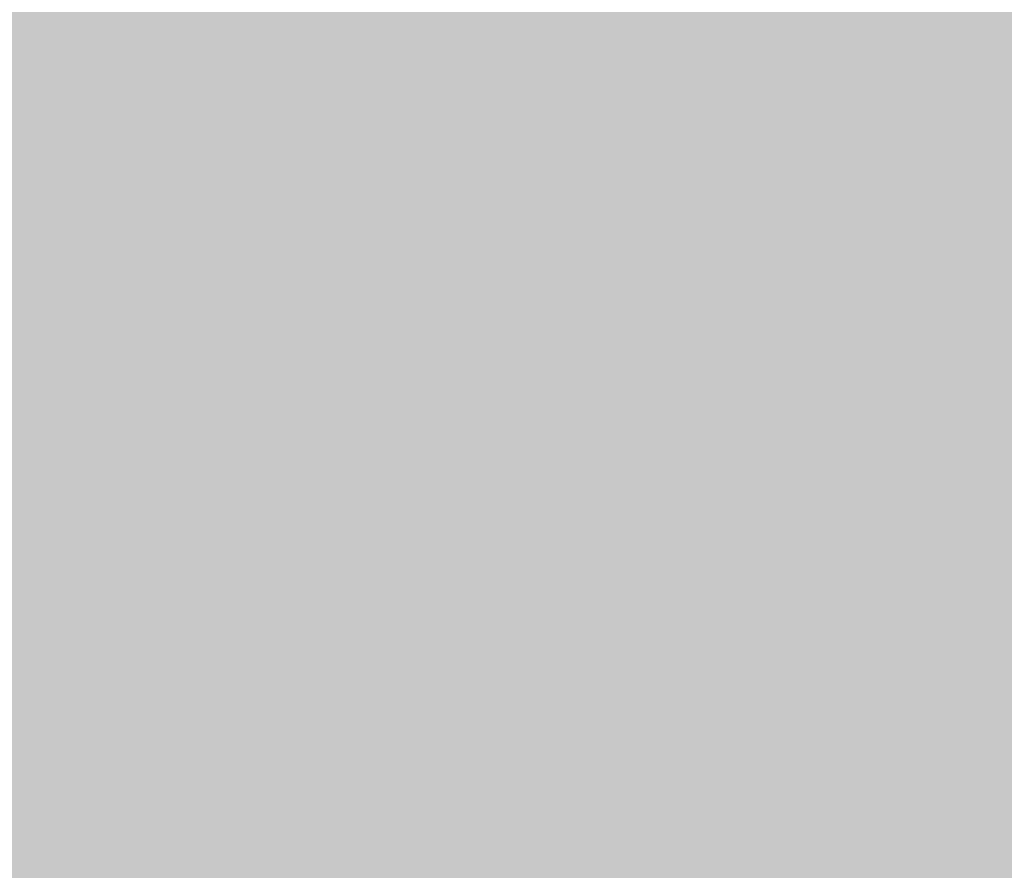
# Model space of a CAD drawing. Units: millimetres. Extents: x -22994 to 29398, y -19990 to 20176.
# Tile 66 of 135: x 225.8137 to 226.3549, y 83.796 to 84.2638. Entities that reach past the tile are written whole.
import ezdxf
from ezdxf import colors
from ezdxf.entities.mleader import LeaderData, LeaderLine
from ezdxf.math import Vec2, Vec3

# ---------------------------------------------------------------- set-up
doc = ezdxf.new("R2010")
doc.units = ezdxf.units.MM
doc.header["$MEASUREMENT"] = 0
for name, color, linetype, lineweight in [('M-ANNO-TEXT', 7, 'Continuous', 25), ('M-DIMS', 2, 'Continuous', 18), ('M-EQPM-PATT', 7, 'Continuous', 18)]:
    doc.layers.add(name, color=color, linetype=linetype, lineweight=lineweight)
doc.styles.get("Standard").update_dxf_attribs({"font": 'arial.ttf'})
doc.dimstyles.get("Standard").update_dxf_attribs({"dimtxt": 0.18, "dimasz": 10000, "dimexe": 0.18, "dimexo": 0.0625, "dimgap": 0.09, "dimtad": 0, "dimtih": 1, "dimtoh": 1, "dimdec": 0, "dimzin": 0, "dimdsep": 46, "dimtxsty": 'Standard', "dimcen": 0.09, "dimadec": 0, "dimazin": 0, "dimtfac": 1, "dimtdec": 0, "dimtofl": 0, "dimtmove": 0, "dimatfit": 3, "dimfxl": 1, "dimtolj": 1, "dimtzin": 0, "dimlwd": 30, "dimarcsym": 0})

# ---------------------------------------------------------------- blocks, each defined once
blk = doc.blocks.new('*D2')
at = {"layer": 'Defpoints', "color": 0, "transparency": 16777216}
for p in [(6.67733, 10.27127), (290.85202, 10.27127), (290.85202, -5.07873)]:
    blk.add_point(p, dxfattribs=at)
at = {"layer": 'M-DIMS', "color": 0, "lineweight": -2, "transparency": 16777216}
for p, q in [((6.67733, 10.20877), (6.67733, -5.25873)), ((290.85202, 10.20877), (290.85202, -5.25873))]:
    blk.add_line(p, q, dxfattribs=at)
at = {"layer": 'M-DIMS', "color": 0, "lineweight": 30, "transparency": 16777216}
for p, q in [((-9993.32267, -5.07873), (-19993.32267, -5.07873)), ((10290.85202, -5.07873), (20290.85202, -5.07873))]:
    blk.add_line(p, q, dxfattribs=at)
at = {"layer": 'M-DIMS', "color": 0, "transparency": 16777216}
for points in [[(-9993.32267, 1661.58794), (-9993.32267, -1671.74539), (6.67733, -5.07873)], [(10290.85202, 1661.58794), (10290.85202, -1671.74539), (290.85202, -5.07873)]]:
    blk.add_solid(points, dxfattribs=at)
at = {"layer": 'M-DIMS', "color": 0, "transparency": 16777216, "insert": (148.76467, -5.07873), "char_height": 0.18, "attachment_point": 5}
blk.add_mtext('\\A1;284.2', dxfattribs=at)
blk = doc.blocks.new('*D3')
at = {"layer": 'Defpoints', "color": 0, "transparency": 16777216}
for p in [(110.26467, 204.16539), (110.26467, 176.36616), (95.83267, 127.96702)]:
    blk.add_point(p, dxfattribs=at)
at = {"layer": 'M-DIMS', "color": 0, "lineweight": -2, "transparency": 16777216}
for p, q in [((95.83267, 128.02952), (95.83267, 204.34539)), ((110.26467, 176.42866), (110.26467, 204.34539))]:
    blk.add_line(p, q, dxfattribs=at)
at = {"layer": 'M-DIMS', "color": 0, "lineweight": 30, "transparency": 16777216}
for p, q in [((-9904.16734, 204.16539), (-19904.16733, 204.16539)), ((10110.26467, 204.16539), (20110.26467, 204.16539))]:
    blk.add_line(p, q, dxfattribs=at)
at = {"layer": 'M-DIMS', "color": 0, "transparency": 16777216}
for points in [[(-9904.16734, 1870.83206), (-9904.16734, -1462.50127), (95.83267, 204.16539)], [(10110.26467, 1870.83206), (10110.26467, -1462.50127), (110.26467, 204.16539)]]:
    blk.add_solid(points, dxfattribs=at)
at = {"layer": 'M-DIMS', "color": 0, "transparency": 16777216, "insert": (103.04867, 204.16539), "char_height": 0.18, "attachment_point": 5}
blk.add_mtext('\\A1;14.432', dxfattribs=at)
blk = doc.blocks.new('*D4')
at = {"layer": 'Defpoints', "color": 0, "transparency": 16777216}
for p in [(116.26467, 204.16539), (110.26467, 176.36616), (116.26467, 176.36616)]:
    blk.add_point(p, dxfattribs=at)
at = {"layer": 'M-DIMS', "color": 0, "lineweight": -2, "transparency": 16777216}
for p, q in [((110.26467, 176.42866), (110.26467, 204.34539)), ((116.26467, 176.42866), (116.26467, 204.34539))]:
    blk.add_line(p, q, dxfattribs=at)
at = {"layer": 'M-DIMS', "color": 0, "lineweight": 30, "transparency": 16777216}
for p, q in [((-9889.73533, 204.16539), (-19889.73533, 204.16539)), ((10116.26467, 204.16539), (20116.26467, 204.16539))]:
    blk.add_line(p, q, dxfattribs=at)
at = {"layer": 'M-DIMS', "color": 0, "transparency": 16777216}
for points in [[(-9889.73533, 1870.83206), (-9889.73533, -1462.50127), (110.26467, 204.16539)], [(10116.26467, 1870.83206), (10116.26467, -1462.50127), (116.26467, 204.16539)]]:
    blk.add_solid(points, dxfattribs=at)
at = {"layer": 'M-DIMS', "color": 0, "transparency": 16777216, "insert": (113.26467, 204.16539), "char_height": 0.18, "attachment_point": 5}
blk.add_mtext('\\A1;6', dxfattribs=at)
blk = doc.blocks.new('*D5')
at = {"layer": 'Defpoints', "color": 0, "transparency": 16777216}
for p in [(181.26467, 204.16539), (116.26467, 176.36616), (181.26467, 176.36616)]:
    blk.add_point(p, dxfattribs=at)
at = {"layer": 'M-DIMS', "color": 0, "lineweight": -2, "transparency": 16777216}
for p, q in [((116.26467, 176.42866), (116.26467, 204.34539)), ((181.26467, 176.42866), (181.26467, 204.34539))]:
    blk.add_line(p, q, dxfattribs=at)
at = {"layer": 'M-DIMS', "color": 0, "lineweight": 30, "transparency": 16777216}
for p, q in [((-9883.73533, 204.16539), (-19883.73533, 204.16539)), ((10181.26467, 204.16539), (20181.26467, 204.16539))]:
    blk.add_line(p, q, dxfattribs=at)
at = {"layer": 'M-DIMS', "color": 0, "transparency": 16777216}
for points in [[(-9883.73533, 1870.83206), (-9883.73533, -1462.50127), (116.26467, 204.16539)], [(10181.26467, 1870.83206), (10181.26467, -1462.50127), (181.26467, 204.16539)]]:
    blk.add_solid(points, dxfattribs=at)
at = {"layer": 'M-DIMS', "color": 0, "transparency": 16777216, "insert": (148.76467, 204.16539), "char_height": 0.18, "attachment_point": 5}
blk.add_mtext('\\A1;65', dxfattribs=at)
blk = doc.blocks.new('*D6')
at = {"layer": 'Defpoints', "color": 0, "transparency": 16777216}
for p in [(187.26467, 204.16539), (181.26467, 176.36616), (187.26467, 176.36616)]:
    blk.add_point(p, dxfattribs=at)
at = {"layer": 'M-DIMS', "color": 0, "lineweight": -2, "transparency": 16777216}
for p, q in [((181.26467, 176.42866), (181.26467, 204.34539)), ((187.26467, 176.42866), (187.26467, 204.34539))]:
    blk.add_line(p, q, dxfattribs=at)
at = {"layer": 'M-DIMS', "color": 0, "lineweight": 30, "transparency": 16777216}
for p, q in [((-9818.73533, 204.16539), (-19818.73533, 204.16539)), ((10187.26467, 204.16539), (20187.26467, 204.16539))]:
    blk.add_line(p, q, dxfattribs=at)
at = {"layer": 'M-DIMS', "color": 0, "transparency": 16777216}
for points in [[(-9818.73533, 1870.83206), (-9818.73533, -1462.50127), (181.26467, 204.16539)], [(10187.26467, 1870.83206), (10187.26467, -1462.50127), (187.26467, 204.16539)]]:
    blk.add_solid(points, dxfattribs=at)
at = {"layer": 'M-DIMS', "color": 0, "transparency": 16777216, "insert": (184.26467, 204.16539), "char_height": 0.18, "attachment_point": 5}
blk.add_mtext('\\A1;6', dxfattribs=at)
blk = doc.blocks.new('*D7')
at = {"layer": 'Defpoints', "color": 0, "transparency": 16777216}
for p in [(201.69668, 204.16539), (187.26467, 176.36616), (201.69668, 127.96702)]:
    blk.add_point(p, dxfattribs=at)
at = {"layer": 'M-DIMS', "color": 0, "lineweight": -2, "transparency": 16777216}
for p, q in [((187.26467, 176.42866), (187.26467, 204.34539)), ((201.69668, 128.02952), (201.69668, 204.34539))]:
    blk.add_line(p, q, dxfattribs=at)
at = {"layer": 'M-DIMS', "color": 0, "lineweight": 30, "transparency": 16777216}
for p, q in [((-9812.73533, 204.16539), (-19812.73533, 204.16539)), ((10201.69668, 204.16539), (20201.69668, 204.16539))]:
    blk.add_line(p, q, dxfattribs=at)
at = {"layer": 'M-DIMS', "color": 0, "transparency": 16777216}
for points in [[(-9812.73533, 1870.83206), (-9812.73533, -1462.50127), (187.26467, 204.16539)], [(10201.69668, 1870.83206), (10201.69668, -1462.50127), (201.69668, 204.16539)]]:
    blk.add_solid(points, dxfattribs=at)
at = {"layer": 'M-DIMS', "color": 0, "transparency": 16777216, "insert": (194.48068, 204.16539), "char_height": 0.18, "attachment_point": 5}
blk.add_mtext('\\A1;14.432', dxfattribs=at)
blk = doc.blocks.new('*D8')
at = {"layer": 'Defpoints', "color": 0, "transparency": 16777216}
for p in [(227.64848, 204.16539), (227.64848, 146.72957), (201.69668, 127.96702)]:
    blk.add_point(p, dxfattribs=at)
at = {"layer": 'M-DIMS', "color": 0, "lineweight": -2, "transparency": 16777216}
for p, q in [((201.69668, 128.02952), (201.69668, 204.34539)), ((227.64848, 146.79207), (227.64848, 204.34539))]:
    blk.add_line(p, q, dxfattribs=at)
at = {"layer": 'M-DIMS', "color": 0, "lineweight": 30, "transparency": 16777216}
for p, q in [((-9798.30332, 204.16539), (-19798.30332, 204.16539)), ((10227.64848, 204.16539), (20227.64848, 204.16539))]:
    blk.add_line(p, q, dxfattribs=at)
at = {"layer": 'M-DIMS', "color": 0, "transparency": 16777216}
for points in [[(-9798.30332, 1870.83206), (-9798.30332, -1462.50127), (201.69668, 204.16539)], [(10227.64848, 1870.83206), (10227.64848, -1462.50127), (227.64848, 204.16539)]]:
    blk.add_solid(points, dxfattribs=at)
at = {"layer": 'M-DIMS', "color": 0, "transparency": 16777216, "insert": (214.67258, 204.16539), "char_height": 0.18, "attachment_point": 5}
blk.add_mtext('\\A1;25.95', dxfattribs=at)
blk = doc.blocks.new('*D9')
at = {"layer": 'Defpoints', "color": 0, "transparency": 16777216}
for p in [(187.26467, 176.36616), (306.20202, 176.36616), (290.85202, 10.27127)]:
    blk.add_point(p, dxfattribs=at)
at = {"layer": 'M-DIMS', "color": 0, "lineweight": 30, "transparency": 16777216}
for p, q in [((306.20202, 10176.36616), (306.20202, 20176.36616)), ((306.20202, -9989.72873), (306.20202, -19989.72873))]:
    blk.add_line(p, q, dxfattribs=at)
at = {"layer": 'M-DIMS', "color": 0, "lineweight": -2, "transparency": 16777216}
for p, q in [((187.32717, 176.36616), (306.38202, 176.36616)), ((290.91452, 10.27127), (306.38202, 10.27127))]:
    blk.add_line(p, q, dxfattribs=at)
at = {"layer": 'M-DIMS', "color": 0, "transparency": 16777216}
for points in [[(-1360.46465, 10176.36616), (1972.86869, 10176.36616), (306.20202, 176.36616)], [(-1360.46465, -9989.72873), (1972.86869, -9989.72873), (306.20202, 10.27127)]]:
    blk.add_solid(points, dxfattribs=at)
at = {"layer": 'M-DIMS', "color": 0, "transparency": 16777216, "insert": (306.20202, 93.31872), "char_height": 0.18, "attachment_point": 5}
blk.add_mtext('\\A1;166.1', dxfattribs=at)
blk = doc.blocks.new('*D10')
at = {"layer": 'Defpoints', "color": 0, "transparency": 16777216}
for p in [(125.64978, 136.0713), (133.34587, 136.0713), (133.34587, -5.07873)]:
    blk.add_point(p, dxfattribs=at)
at = {"layer": 'M-DIMS', "color": 0, "lineweight": -2, "transparency": 16777216}
for p, q in [((125.64978, 136.0088), (125.64978, -5.25872)), ((133.34587, 136.0088), (133.34587, -5.25872))]:
    blk.add_line(p, q, dxfattribs=at)
at = {"layer": 'M-DIMS', "color": 0, "lineweight": 30, "transparency": 16777216}
for p, q in [((-9874.35022, -5.07873), (-19874.35022, -5.07873)), ((10133.34587, -5.07873), (20133.34587, -5.07873))]:
    blk.add_line(p, q, dxfattribs=at)
at = {"layer": 'M-DIMS', "color": 0, "transparency": 16777216}
for points in [[(-9874.35022, 1661.58794), (-9874.35022, -1671.74539), (125.64978, -5.07873)], [(10133.34587, 1661.58794), (10133.34587, -1671.74539), (133.34587, -5.07873)]]:
    blk.add_solid(points, dxfattribs=at)
at = {"layer": 'M-DIMS', "color": 0, "transparency": 16777216, "insert": (129.49783, -5.07873), "char_height": 0.18, "attachment_point": 5}
blk.add_mtext('\\A1;7.696', dxfattribs=at)
blk = doc.blocks.new('*D11')
at = {"layer": 'Defpoints', "color": 0, "transparency": 16777216}
for p in [(133.34587, 136.0713), (135.64978, 136.0713), (135.64978, -5.07873)]:
    blk.add_point(p, dxfattribs=at)
at = {"layer": 'M-DIMS', "color": 0, "lineweight": -2, "transparency": 16777216}
for p, q in [((133.34587, 136.0088), (133.34587, -5.25872)), ((135.64978, 136.0088), (135.64978, -5.25872))]:
    blk.add_line(p, q, dxfattribs=at)
at = {"layer": 'M-DIMS', "color": 0, "lineweight": 30, "transparency": 16777216}
for p, q in [((-9866.65413, -5.07873), (-19866.65413, -5.07873)), ((10135.64978, -5.07873), (20135.64978, -5.07873))]:
    blk.add_line(p, q, dxfattribs=at)
at = {"layer": 'M-DIMS', "color": 0, "transparency": 16777216}
for points in [[(-9866.65413, 1661.58794), (-9866.65413, -1671.74539), (133.34587, -5.07873)], [(10135.64978, 1661.58794), (10135.64978, -1671.74539), (135.64978, -5.07873)]]:
    blk.add_solid(points, dxfattribs=at)
at = {"layer": 'M-DIMS', "color": 0, "transparency": 16777216, "insert": (134.49783, -5.07873), "char_height": 0.18, "attachment_point": 5}
blk.add_mtext('\\A1;2.304', dxfattribs=at)
blk = doc.blocks.new('*D12')
at = {"layer": 'Defpoints', "color": 0, "transparency": 16777216}
for p in [(135.64978, 136.0713), (145.64978, 136.0713), (145.64978, -5.07873)]:
    blk.add_point(p, dxfattribs=at)
at = {"layer": 'M-DIMS', "color": 0, "lineweight": -2, "transparency": 16777216}
for p, q in [((135.64978, 136.0088), (135.64978, -5.25872)), ((145.64978, 136.0088), (145.64978, -5.25872))]:
    blk.add_line(p, q, dxfattribs=at)
at = {"layer": 'M-DIMS', "color": 0, "lineweight": 30, "transparency": 16777216}
for p, q in [((-9864.35022, -5.07873), (-19864.35022, -5.07873)), ((10145.64978, -5.07873), (20145.64978, -5.07873))]:
    blk.add_line(p, q, dxfattribs=at)
at = {"layer": 'M-DIMS', "color": 0, "transparency": 16777216}
for points in [[(-9864.35022, 1661.58794), (-9864.35022, -1671.74539), (135.64978, -5.07873)], [(10145.64978, 1661.58794), (10145.64978, -1671.74539), (145.64978, -5.07873)]]:
    blk.add_solid(points, dxfattribs=at)
at = {"layer": 'M-DIMS', "color": 0, "transparency": 16777216, "insert": (140.64978, -5.07873), "char_height": 0.18, "attachment_point": 5}
blk.add_mtext('\\A1;10', dxfattribs=at)
blk = doc.blocks.new('*D13')
at = {"layer": 'Defpoints', "color": 0, "transparency": 16777216}
for p in [(145.64978, 136.0713), (155.64978, 136.0713), (155.64978, -5.07873)]:
    blk.add_point(p, dxfattribs=at)
at = {"layer": 'M-DIMS', "color": 0, "lineweight": -2, "transparency": 16777216}
for p, q in [((145.64978, 136.0088), (145.64978, -5.25872)), ((155.64978, 136.0088), (155.64978, -5.25872))]:
    blk.add_line(p, q, dxfattribs=at)
at = {"layer": 'M-DIMS', "color": 0, "lineweight": 30, "transparency": 16777216}
for p, q in [((-9854.35022, -5.07873), (-19854.35022, -5.07873)), ((10155.64978, -5.07873), (20155.64978, -5.07873))]:
    blk.add_line(p, q, dxfattribs=at)
at = {"layer": 'M-DIMS', "color": 0, "transparency": 16777216}
for points in [[(-9854.35022, 1661.58794), (-9854.35022, -1671.74539), (145.64978, -5.07873)], [(10155.64978, 1661.58794), (10155.64978, -1671.74539), (155.64978, -5.07873)]]:
    blk.add_solid(points, dxfattribs=at)
at = {"layer": 'M-DIMS', "color": 0, "transparency": 16777216, "insert": (150.64978, -5.07873), "char_height": 0.18, "attachment_point": 5}
blk.add_mtext('\\A1;10', dxfattribs=at)
blk = doc.blocks.new('*D14')
at = {"layer": 'Defpoints', "color": 0, "transparency": 16777216}
for p in [(155.64978, 136.0713), (165.64978, 136.0713), (165.64978, -5.07873)]:
    blk.add_point(p, dxfattribs=at)
at = {"layer": 'M-DIMS', "color": 0, "lineweight": -2, "transparency": 16777216}
for p, q in [((155.64978, 136.0088), (155.64978, -5.25872)), ((165.64978, 136.0088), (165.64978, -5.25872))]:
    blk.add_line(p, q, dxfattribs=at)
at = {"layer": 'M-DIMS', "color": 0, "lineweight": 30, "transparency": 16777216}
for p, q in [((-9844.35022, -5.07873), (-19844.35022, -5.07873)), ((10165.64978, -5.07873), (20165.64978, -5.07873))]:
    blk.add_line(p, q, dxfattribs=at)
at = {"layer": 'M-DIMS', "color": 0, "transparency": 16777216}
for points in [[(-9844.35022, 1661.58794), (-9844.35022, -1671.74539), (155.64978, -5.07873)], [(10165.64978, 1661.58794), (10165.64978, -1671.74539), (165.64978, -5.07873)]]:
    blk.add_solid(points, dxfattribs=at)
at = {"layer": 'M-DIMS', "color": 0, "transparency": 16777216, "insert": (160.64978, -5.07873), "char_height": 0.18, "attachment_point": 5}
blk.add_mtext('\\A1;10', dxfattribs=at)
blk = doc.blocks.new('*D15')
at = {"layer": 'Defpoints', "color": 0, "transparency": 16777216}
for p in [(173.34587, 154.78801), (173.34587, 136.0713), (306.20202, 136.0713)]:
    blk.add_point(p, dxfattribs=at)
at = {"layer": 'M-DIMS', "color": 0, "lineweight": 30, "transparency": 16777216}
for p, q in [((306.20202, 10154.78801), (306.20202, 20154.78801)), ((306.20202, -9863.9287), (306.20202, -19863.9287))]:
    blk.add_line(p, q, dxfattribs=at)
at = {"layer": 'M-DIMS', "color": 0, "lineweight": -2, "transparency": 16777216}
for p, q in [((173.40837, 154.78801), (306.38202, 154.78801)), ((173.40837, 136.0713), (306.38202, 136.0713))]:
    blk.add_line(p, q, dxfattribs=at)
at = {"layer": 'M-DIMS', "color": 0, "transparency": 16777216}
for points in [[(-1360.46465, 10154.78801), (1972.86869, 10154.78801), (306.20202, 154.78801)], [(-1360.46465, -9863.9287), (1972.86869, -9863.9287), (306.20202, 136.0713)]]:
    blk.add_solid(points, dxfattribs=at)
at = {"layer": 'M-DIMS', "color": 0, "transparency": 16777216, "insert": (306.20202, 145.42965), "char_height": 0.18, "attachment_point": 5}
blk.add_mtext('\\A1;18.717', dxfattribs=at)
blk = doc.blocks.new('*D16')
at = {"layer": 'Defpoints', "color": 0, "transparency": 16777216}
for p in [(120.17023, 204.16539), (110.46575, 48.03494), (120.17023, 48.03494)]:
    blk.add_point(p, dxfattribs=at)
at = {"layer": 'M-DIMS', "color": 0, "lineweight": -2, "transparency": 16777216}
for p, q in [((110.46575, 48.09744), (110.46575, 204.34539)), ((120.17023, 48.09744), (120.17023, 204.34539))]:
    blk.add_line(p, q, dxfattribs=at)
at = {"layer": 'M-DIMS', "color": 0, "lineweight": 30, "transparency": 16777216}
for p, q in [((-9889.53425, 204.16539), (-19889.53425, 204.16539)), ((10120.17023, 204.16539), (20120.17023, 204.16539))]:
    blk.add_line(p, q, dxfattribs=at)
at = {"layer": 'M-DIMS', "color": 0, "transparency": 16777216}
for points in [[(-9889.53425, 1870.83206), (-9889.53425, -1462.50127), (110.46575, 204.16539)], [(10120.17023, 1870.83206), (10120.17023, -1462.50127), (120.17023, 204.16539)]]:
    blk.add_solid(points, dxfattribs=at)
at = {"layer": 'M-DIMS', "color": 0, "transparency": 16777216, "insert": (115.31799, 204.16539), "char_height": 0.18, "attachment_point": 5}
blk.add_mtext('\\A1;9.704', dxfattribs=at)
blk = doc.blocks.new('*D17')
at = {"layer": 'Defpoints', "color": 0, "transparency": 16777216}
for p in [(126.17023, 204.16539), (120.17023, 48.03494), (126.17023, 48.03494)]:
    blk.add_point(p, dxfattribs=at)
at = {"layer": 'M-DIMS', "color": 0, "lineweight": -2, "transparency": 16777216}
for p, q in [((120.17023, 48.09744), (120.17023, 204.34539)), ((126.17023, 48.09744), (126.17023, 204.34539))]:
    blk.add_line(p, q, dxfattribs=at)
at = {"layer": 'M-DIMS', "color": 0, "lineweight": 30, "transparency": 16777216}
for p, q in [((-9879.82977, 204.16539), (-19879.82977, 204.16539)), ((10126.17023, 204.16539), (20126.17023, 204.16539))]:
    blk.add_line(p, q, dxfattribs=at)
at = {"layer": 'M-DIMS', "color": 0, "transparency": 16777216}
for points in [[(-9879.82977, 1870.83206), (-9879.82977, -1462.50127), (120.17023, 204.16539)], [(10126.17023, 1870.83206), (10126.17023, -1462.50127), (126.17023, 204.16539)]]:
    blk.add_solid(points, dxfattribs=at)
at = {"layer": 'M-DIMS', "color": 0, "transparency": 16777216, "insert": (123.17023, 204.16539), "char_height": 0.18, "attachment_point": 5}
blk.add_mtext('\\A1;6', dxfattribs=at)
blk = doc.blocks.new('*D18')
at = {"layer": 'Defpoints', "color": 0, "transparency": 16777216}
for p in [(132.17023, 204.16539), (126.17023, 48.03494), (132.17023, 48.03494)]:
    blk.add_point(p, dxfattribs=at)
at = {"layer": 'M-DIMS', "color": 0, "lineweight": -2, "transparency": 16777216}
for p, q in [((126.17023, 48.09744), (126.17023, 204.34539)), ((132.17023, 48.09744), (132.17023, 204.34539))]:
    blk.add_line(p, q, dxfattribs=at)
at = {"layer": 'M-DIMS', "color": 0, "lineweight": 30, "transparency": 16777216}
for p, q in [((-9873.82977, 204.16539), (-19873.82977, 204.16539)), ((10132.17023, 204.16539), (20132.17023, 204.16539))]:
    blk.add_line(p, q, dxfattribs=at)
at = {"layer": 'M-DIMS', "color": 0, "transparency": 16777216}
for points in [[(-9873.82977, 1870.83206), (-9873.82977, -1462.50127), (126.17023, 204.16539)], [(10132.17023, 1870.83206), (10132.17023, -1462.50127), (132.17023, 204.16539)]]:
    blk.add_solid(points, dxfattribs=at)
at = {"layer": 'M-DIMS', "color": 0, "transparency": 16777216, "insert": (129.17023, 204.16539), "char_height": 0.18, "attachment_point": 5}
blk.add_mtext('\\A1;6', dxfattribs=at)
blk = doc.blocks.new('*D19')
at = {"layer": 'Defpoints', "color": 0, "transparency": 16777216}
for p in [(138.17023, 204.16539), (132.17023, 48.03494), (138.17023, 48.03494)]:
    blk.add_point(p, dxfattribs=at)
at = {"layer": 'M-DIMS', "color": 0, "lineweight": -2, "transparency": 16777216}
for p, q in [((132.17023, 48.09744), (132.17023, 204.34539)), ((138.17023, 48.09744), (138.17023, 204.34539))]:
    blk.add_line(p, q, dxfattribs=at)
at = {"layer": 'M-DIMS', "color": 0, "lineweight": 30, "transparency": 16777216}
for p, q in [((-9867.82977, 204.16539), (-19867.82977, 204.16539)), ((10138.17023, 204.16539), (20138.17023, 204.16539))]:
    blk.add_line(p, q, dxfattribs=at)
at = {"layer": 'M-DIMS', "color": 0, "transparency": 16777216}
for points in [[(-9867.82977, 1870.83206), (-9867.82977, -1462.50127), (132.17023, 204.16539)], [(10138.17023, 1870.83206), (10138.17023, -1462.50127), (138.17023, 204.16539)]]:
    blk.add_solid(points, dxfattribs=at)
at = {"layer": 'M-DIMS', "color": 0, "transparency": 16777216, "insert": (135.17023, 204.16539), "char_height": 0.18, "attachment_point": 5}
blk.add_mtext('\\A1;6', dxfattribs=at)
blk = doc.blocks.new('*D20')
at = {"layer": 'Defpoints', "color": 0, "transparency": 16777216}
for p in [(144.17023, 204.16539), (138.17023, 48.03494), (144.17023, 48.03494)]:
    blk.add_point(p, dxfattribs=at)
at = {"layer": 'M-DIMS', "color": 0, "lineweight": -2, "transparency": 16777216}
for p, q in [((138.17023, 48.09744), (138.17023, 204.34539)), ((144.17023, 48.09744), (144.17023, 204.34539))]:
    blk.add_line(p, q, dxfattribs=at)
at = {"layer": 'M-DIMS', "color": 0, "lineweight": 30, "transparency": 16777216}
for p, q in [((-9861.82977, 204.16539), (-19861.82977, 204.16539)), ((10144.17023, 204.16539), (20144.17023, 204.16539))]:
    blk.add_line(p, q, dxfattribs=at)
at = {"layer": 'M-DIMS', "color": 0, "transparency": 16777216}
for points in [[(-9861.82977, 1870.83206), (-9861.82977, -1462.50127), (138.17023, 204.16539)], [(10144.17023, 1870.83206), (10144.17023, -1462.50127), (144.17023, 204.16539)]]:
    blk.add_solid(points, dxfattribs=at)
at = {"layer": 'M-DIMS', "color": 0, "transparency": 16777216, "insert": (141.17023, 204.16539), "char_height": 0.18, "attachment_point": 5}
blk.add_mtext('\\A1;6', dxfattribs=at)
blk = doc.blocks.new('*D21')
at = {"layer": 'Defpoints', "color": 0, "transparency": 16777216}
for p in [(149.11567, 204.16539), (144.17023, 48.03494), (149.11567, 48.03494)]:
    blk.add_point(p, dxfattribs=at)
at = {"layer": 'M-DIMS', "color": 0, "lineweight": -2, "transparency": 16777216}
for p, q in [((144.17023, 48.09744), (144.17023, 204.34539)), ((149.11567, 48.09744), (149.11567, 204.34539))]:
    blk.add_line(p, q, dxfattribs=at)
at = {"layer": 'M-DIMS', "color": 0, "lineweight": 30, "transparency": 16777216}
for p, q in [((-9855.82977, 204.16539), (-19855.82977, 204.16539)), ((10149.11567, 204.16539), (20149.11567, 204.16539))]:
    blk.add_line(p, q, dxfattribs=at)
at = {"layer": 'M-DIMS', "color": 0, "transparency": 16777216}
for points in [[(-9855.82977, 1870.83206), (-9855.82977, -1462.50127), (144.17023, 204.16539)], [(10149.11567, 1870.83206), (10149.11567, -1462.50127), (149.11567, 204.16539)]]:
    blk.add_solid(points, dxfattribs=at)
at = {"layer": 'M-DIMS', "color": 0, "transparency": 16777216, "insert": (146.64295, 204.16539), "char_height": 0.18, "attachment_point": 5}
blk.add_mtext('\\A1;4.945', dxfattribs=at)
blk = doc.blocks.new('*D22')
at = {"layer": 'Defpoints', "color": 0, "transparency": 16777216}
for p in [(149.11567, 30.98952), (155.11567, 30.98952), (155.11567, -5.07873)]:
    blk.add_point(p, dxfattribs=at)
at = {"layer": 'M-DIMS', "color": 0, "lineweight": -2, "transparency": 16777216}
for p, q in [((149.11567, 30.92702), (149.11567, -5.25872)), ((155.11567, 30.92702), (155.11567, -5.25872))]:
    blk.add_line(p, q, dxfattribs=at)
at = {"layer": 'M-DIMS', "color": 0, "lineweight": 30, "transparency": 16777216}
for p, q in [((-9850.88433, -5.07873), (-19850.88433, -5.07873)), ((10155.11567, -5.07873), (20155.11567, -5.07873))]:
    blk.add_line(p, q, dxfattribs=at)
at = {"layer": 'M-DIMS', "color": 0, "transparency": 16777216}
for points in [[(-9850.88433, 1661.58794), (-9850.88433, -1671.74539), (149.11567, -5.07873)], [(10155.11567, 1661.58794), (10155.11567, -1671.74539), (155.11567, -5.07873)]]:
    blk.add_solid(points, dxfattribs=at)
at = {"layer": 'M-DIMS', "color": 0, "transparency": 16777216, "insert": (152.11567, -5.07873), "char_height": 0.18, "attachment_point": 5}
blk.add_mtext('\\A1;6', dxfattribs=at)
blk = doc.blocks.new('*D23')
at = {"layer": 'Defpoints', "color": 0, "transparency": 16777216}
for p in [(155.11567, 30.98952), (161.11567, 30.98952), (161.11567, -5.07873)]:
    blk.add_point(p, dxfattribs=at)
at = {"layer": 'M-DIMS', "color": 0, "lineweight": -2, "transparency": 16777216}
for p, q in [((155.11567, 30.92702), (155.11567, -5.25872)), ((161.11567, 30.92702), (161.11567, -5.25872))]:
    blk.add_line(p, q, dxfattribs=at)
at = {"layer": 'M-DIMS', "color": 0, "lineweight": 30, "transparency": 16777216}
for p, q in [((-9844.88433, -5.07873), (-19844.88433, -5.07873)), ((10161.11567, -5.07873), (20161.11567, -5.07873))]:
    blk.add_line(p, q, dxfattribs=at)
at = {"layer": 'M-DIMS', "color": 0, "transparency": 16777216}
for points in [[(-9844.88433, 1661.58794), (-9844.88433, -1671.74539), (155.11567, -5.07873)], [(10161.11567, 1661.58794), (10161.11567, -1671.74539), (161.11567, -5.07873)]]:
    blk.add_solid(points, dxfattribs=at)
at = {"layer": 'M-DIMS', "color": 0, "transparency": 16777216, "insert": (158.11567, -5.07873), "char_height": 0.18, "attachment_point": 5}
blk.add_mtext('\\A1;6', dxfattribs=at)
blk = doc.blocks.new('*D24')
at = {"layer": 'Defpoints', "color": 0, "transparency": 16777216}
for p in [(161.11567, 30.98952), (166.43874, 30.98952), (166.43874, -5.07873)]:
    blk.add_point(p, dxfattribs=at)
at = {"layer": 'M-DIMS', "color": 0, "lineweight": -2, "transparency": 16777216}
for p, q in [((161.11567, 30.92702), (161.11567, -5.25872)), ((166.43874, 30.92702), (166.43874, -5.25872))]:
    blk.add_line(p, q, dxfattribs=at)
at = {"layer": 'M-DIMS', "color": 0, "lineweight": 30, "transparency": 16777216}
for p, q in [((-9838.88433, -5.07873), (-19838.88433, -5.07873)), ((10166.43874, -5.07873), (20166.43874, -5.07873))]:
    blk.add_line(p, q, dxfattribs=at)
at = {"layer": 'M-DIMS', "color": 0, "transparency": 16777216}
for points in [[(-9838.88433, 1661.58794), (-9838.88433, -1671.74539), (161.11567, -5.07873)], [(10166.43874, 1661.58794), (10166.43874, -1671.74539), (166.43874, -5.07873)]]:
    blk.add_solid(points, dxfattribs=at)
at = {"layer": 'M-DIMS', "color": 0, "transparency": 16777216, "insert": (163.7772, -5.07873), "char_height": 0.18, "attachment_point": 5}
blk.add_mtext('\\A1;5.323', dxfattribs=at)
blk = doc.blocks.new('*D25')
at = {"layer": 'Defpoints', "color": 0, "transparency": 16777216}
for p in [(166.43874, 30.98952), (172.43874, 30.98952), (172.43874, -5.07873)]:
    blk.add_point(p, dxfattribs=at)
at = {"layer": 'M-DIMS', "color": 0, "lineweight": -2, "transparency": 16777216}
for p, q in [((166.43874, 30.92702), (166.43874, -5.25872)), ((172.43874, 30.92702), (172.43874, -5.25872))]:
    blk.add_line(p, q, dxfattribs=at)
at = {"layer": 'M-DIMS', "color": 0, "lineweight": 30, "transparency": 16777216}
for p, q in [((-9833.56126, -5.07873), (-19833.56126, -5.07873)), ((10172.43874, -5.07873), (20172.43874, -5.07873))]:
    blk.add_line(p, q, dxfattribs=at)
at = {"layer": 'M-DIMS', "color": 0, "transparency": 16777216}
for points in [[(-9833.56126, 1661.58794), (-9833.56126, -1671.74539), (166.43874, -5.07873)], [(10172.43874, 1661.58794), (10172.43874, -1671.74539), (172.43874, -5.07873)]]:
    blk.add_solid(points, dxfattribs=at)
at = {"layer": 'M-DIMS', "color": 0, "transparency": 16777216, "insert": (169.43874, -5.07873), "char_height": 0.18, "attachment_point": 5}
blk.add_mtext('\\A1;6', dxfattribs=at)
blk = doc.blocks.new('*D26')
at = {"layer": 'Defpoints', "color": 0, "transparency": 16777216}
for p in [(172.43874, 30.98952), (178.43874, 30.98952), (178.43874, -5.07873)]:
    blk.add_point(p, dxfattribs=at)
at = {"layer": 'M-DIMS', "color": 0, "lineweight": -2, "transparency": 16777216}
for p, q in [((172.43874, 30.92702), (172.43874, -5.25872)), ((178.43874, 30.92702), (178.43874, -5.25872))]:
    blk.add_line(p, q, dxfattribs=at)
at = {"layer": 'M-DIMS', "color": 0, "lineweight": 30, "transparency": 16777216}
for p, q in [((-9827.56126, -5.07873), (-19827.56126, -5.07873)), ((10178.43874, -5.07873), (20178.43874, -5.07873))]:
    blk.add_line(p, q, dxfattribs=at)
at = {"layer": 'M-DIMS', "color": 0, "transparency": 16777216}
for points in [[(-9827.56126, 1661.58794), (-9827.56126, -1671.74539), (172.43874, -5.07873)], [(10178.43874, 1661.58794), (10178.43874, -1671.74539), (178.43874, -5.07873)]]:
    blk.add_solid(points, dxfattribs=at)
at = {"layer": 'M-DIMS', "color": 0, "transparency": 16777216, "insert": (175.43874, -5.07873), "char_height": 0.18, "attachment_point": 5}
blk.add_mtext('\\A1;6', dxfattribs=at)
blk = doc.blocks.new('*D27')
at = {"layer": 'Defpoints', "color": 0, "transparency": 16777216}
for p in [(178.43874, 30.98952), (188.11747, 30.98952), (188.11747, -5.07873)]:
    blk.add_point(p, dxfattribs=at)
at = {"layer": 'M-DIMS', "color": 0, "lineweight": -2, "transparency": 16777216}
for p, q in [((178.43874, 30.92702), (178.43874, -5.25872)), ((188.11747, 30.92702), (188.11747, -5.25872))]:
    blk.add_line(p, q, dxfattribs=at)
at = {"layer": 'M-DIMS', "color": 0, "lineweight": 30, "transparency": 16777216}
for p, q in [((-9821.56126, -5.07873), (-19821.56126, -5.07873)), ((10188.11747, -5.07873), (20188.11747, -5.07873))]:
    blk.add_line(p, q, dxfattribs=at)
at = {"layer": 'M-DIMS', "color": 0, "transparency": 16777216}
for points in [[(-9821.56126, 1661.58794), (-9821.56126, -1671.74539), (178.43874, -5.07873)], [(10188.11747, 1661.58794), (10188.11747, -1671.74539), (188.11747, -5.07873)]]:
    blk.add_solid(points, dxfattribs=at)
at = {"layer": 'M-DIMS', "color": 0, "transparency": 16777216, "insert": (183.27811, -5.07873), "char_height": 0.18, "attachment_point": 5}
blk.add_mtext('\\A1;9.679', dxfattribs=at)
blk = doc.blocks.new('*D28')
at = {"layer": 'Defpoints', "color": 0, "transparency": 16777216}
for p in [(188.11747, 48.03494), (306.20202, 48.03494), (188.11747, 30.98952)]:
    blk.add_point(p, dxfattribs=at)
at = {"layer": 'M-DIMS', "color": 0, "lineweight": 30, "transparency": 16777216}
for p, q in [((306.20202, 10048.03494), (306.20202, 20048.03494)), ((306.20202, -9969.01048), (306.20202, -19969.01048))]:
    blk.add_line(p, q, dxfattribs=at)
at = {"layer": 'M-DIMS', "color": 0, "lineweight": -2, "transparency": 16777216}
for p, q in [((188.17997, 48.03494), (306.38202, 48.03494)), ((188.17997, 30.98952), (306.38202, 30.98952))]:
    blk.add_line(p, q, dxfattribs=at)
at = {"layer": 'M-DIMS', "color": 0, "transparency": 16777216}
for points in [[(-1360.46465, 10048.03494), (1972.86869, 10048.03494), (306.20202, 48.03494)], [(-1360.46465, -9969.01048), (1972.86869, -9969.01048), (306.20202, 30.98952)]]:
    blk.add_solid(points, dxfattribs=at)
at = {"layer": 'M-DIMS', "color": 0, "transparency": 16777216, "insert": (306.20202, 39.51223), "char_height": 0.18, "attachment_point": 5}
blk.add_mtext('\\A1;17.045', dxfattribs=at)
blk = doc.blocks.new('*D29')
at = {"layer": 'Defpoints', "color": 0, "transparency": 16777216}
for p in [(36.80064, 80.04502), (64.02964, 80.045)]:
    blk.add_point(p, dxfattribs=at)
at = {"layer": 'M-DIMS', "color": 0, "lineweight": -2, "transparency": 16777216}
for p, q in [((50.41514, 79.95501), (50.41514, 80.13501)), ((50.32514, 80.04501), (50.50514, 80.04501))]:
    blk.add_line(p, q, dxfattribs=at)
at = {"layer": 'M-DIMS', "color": 0, "lineweight": 30, "transparency": 16777216}
blk.add_line((20064.02964, 80.03031), (10064.02964, 80.03765), dxfattribs=at)
at = {"layer": 'M-DIMS', "color": 0, "transparency": 16777216}
blk.add_solid([(10064.03087, 1746.70432), (10064.02842, -1586.62901), (64.02964, 80.045)], dxfattribs=at)
at = {"layer": 'M-DIMS', "color": 0, "transparency": 16777216, "insert": (20064.52126, 80.03031), "char_height": 0.18, "attachment_point": 5}
blk.add_mtext('\\A1;∅27.23', dxfattribs=at)
blk = doc.blocks.new('*D30')
at = {"layer": 'Defpoints', "color": 0, "transparency": 16777216}
for p in [(216.31485, 146.72913), (238.98211, 146.73)]:
    blk.add_point(p, dxfattribs=at)
at = {"layer": 'M-DIMS', "color": 0, "lineweight": 30, "transparency": 16777216}
blk.add_line((20238.9821, 147.49586), (10238.98211, 147.11293), dxfattribs=at)
at = {"layer": 'M-DIMS', "color": 0, "lineweight": -2, "transparency": 16777216}
for p, q in [((227.64848, 146.63957), (227.64848, 146.81957)), ((227.55848, 146.72957), (227.73848, 146.72957))]:
    blk.add_line(p, q, dxfattribs=at)
at = {"layer": 'M-DIMS', "color": 0, "transparency": 16777216}
blk.add_solid([(10238.91828, 1813.7796), (10239.04593, -1519.55373), (238.98211, 146.73)], dxfattribs=at)
at = {"layer": 'M-DIMS', "color": 0, "transparency": 16777216, "insert": (20239.54365, 147.49586), "char_height": 0.18, "attachment_point": 5}
blk.add_mtext('\\A1;∅22.667', dxfattribs=at)
blk = doc.blocks.new('*D31')
at = {"layer": 'Defpoints', "color": 0, "transparency": 16777216}
for p in [(223.16413, 146.72913), (232.13283, 146.73)]:
    blk.add_point(p, dxfattribs=at)
at = {"layer": 'M-DIMS', "color": 0, "lineweight": 30, "transparency": 16777216}
blk.add_line((20232.13273, 148.66562), (10232.13278, 147.69781), dxfattribs=at)
at = {"layer": 'M-DIMS', "color": 0, "lineweight": -2, "transparency": 16777216}
for p, q in [((227.64848, 146.63957), (227.64848, 146.81957)), ((227.55848, 146.72957), (227.73848, 146.72957))]:
    blk.add_line(p, q, dxfattribs=at)
at = {"layer": 'M-DIMS', "color": 0, "transparency": 16777216}
blk.add_solid([(10231.97148, 1814.36447), (10232.29408, -1518.96885), (232.13283, 146.73)], dxfattribs=at)
at = {"layer": 'M-DIMS', "color": 0, "transparency": 16777216, "insert": (20232.62454, 148.66562), "char_height": 0.18, "attachment_point": 5}
blk.add_mtext('\\A1;∅8.969', dxfattribs=at)

msp = doc.modelspace()

# ---------------------------------------------------------------- hatches: boundary and pattern name
at = {"layer": 'M-EQPM-PATT'}
h = msp.add_hatch(color=256, dxfattribs=at)
h.set_gradient(color1=(205, 32, 39), color2=(205, 32, 39), tint=1)
h.paths.add_polyline_path([(116.26467, 150.36616), (116.26467, 170.36616), (116.26467, 176.36616), (110.26467, 176.36616), (110.26467, 152.02763), (95.83267, 127.96702), (95.83267, 16.60628), (201.69668, 16.60628), (201.69668, 127.96702), (187.26467, 152.02763), (187.26467, 176.36616), (181.26467, 176.36616), (181.26467, 170.36616), (181.26467, 150.36616), (195.69668, 126.30555), (195.69668, 22.60628), (101.83267, 22.60628), (101.83267, 126.30555)])
h.paths.add_polyline_path([(185.22083, 88.63474), (101.83267, 88.63474), (101.83267, 87.63474), (182.80661, 87.63474), (178.73126, 83.55939), (195.69668, 83.55939), (195.69668, 84.55939), (181.14547, 84.55939)], flags=17)
h.paths.add_polyline_path([(95.83267, 88.63474), (60.97786, 88.63474, -0.022855), (61.71782, 87.63474), (95.83267, 87.63474)])
h.paths.add_polyline_path([(215.62123, 86.51891), (215.62123, 80.59986), (220.50954, 83.55939)])
h.paths.add_polyline_path([(215.62123, 84.55939), (201.69668, 84.55939), (201.69668, 83.55939), (215.62123, 83.55939)])
h.paths.add_polyline_path([(225.39784, 86.51891), (220.50954, 83.55939), (225.39784, 80.59986)])
h.paths.add_polyline_path([(231.62561, 84.55939), (225.39784, 84.55939), (225.39784, 83.55939), (231.62561, 83.55939)])

# ---------------------------------------------------------------- dimensions: what is measured, and where the dimension line sits
at = {"layer": 'M-DIMS'}
for base, p1, p2, override, picture, middle in [((306.20202, 176.36616), (290.85202, 10.27127), (187.26467, 176.36616), {"dimdec": 1, "dimlfac": 1, "dimrnd": 0, "dimzin": 0, "dimdsep": 46, "dimlunit": 2}, '*D9', (306.20202, 93.31872)), ((306.20202, 136.0713), (173.34587, 154.78801), (173.34587, 136.0713), {"dimdec": 3, "dimlfac": 1, "dimrnd": 0, "dimzin": 0, "dimdsep": 46, "dimlunit": 2}, '*D15', (306.20202, 145.42965)), ((306.20202, 48.03494), (188.11747, 30.98952), (188.11747, 48.03494), {"dimdec": 3, "dimlfac": 1, "dimrnd": 0, "dimzin": 0, "dimdsep": 46, "dimlunit": 2}, '*D28', (306.20202, 39.51223))]:
    dim = msp.add_linear_dim(base=base, p1=p1, p2=p2, angle=90, dimstyle='Standard', override=override, dxfattribs=at)
    dim.commit()
    dim.dimension.update_dxf_attribs({"geometry": picture, "text_midpoint": middle})
for base, p1, p2, override, picture, middle in [((110.26467, 204.16539), (95.83267, 127.96702), (110.26467, 176.36616), {"dimdec": 3, "dimlfac": 1, "dimrnd": 0, "dimzin": 0, "dimdsep": 46, "dimlunit": 2}, '*D3', (103.04867, 204.16539)), ((116.26467, 204.16539), (110.26467, 176.36616), (116.26467, 176.36616), {"dimdec": 0, "dimlfac": 1, "dimrnd": 0, "dimzin": 0, "dimdsep": 46, "dimlunit": 2}, '*D4', (113.26467, 204.16539)), ((120.17023, 204.16539), (110.46575, 48.03494), (120.17023, 48.03494), {"dimdec": 3, "dimlfac": 1, "dimrnd": 0, "dimzin": 0, "dimdsep": 46, "dimlunit": 2}, '*D16', (115.31799, 204.16539)), ((181.26467, 204.16539), (116.26467, 176.36616), (181.26467, 176.36616), {"dimdec": 0, "dimlfac": 1, "dimrnd": 0, "dimzin": 0, "dimdsep": 46, "dimlunit": 2}, '*D5', (148.76467, 204.16539)), ((126.17023, 204.16539), (120.17023, 48.03494), (126.17023, 48.03494), {"dimdec": 0, "dimlfac": 1, "dimrnd": 0, "dimzin": 0, "dimdsep": 46, "dimlunit": 2}, '*D17', (123.17023, 204.16539)), ((132.17023, 204.16539), (126.17023, 48.03494), (132.17023, 48.03494), {"dimdec": 0, "dimlfac": 1, "dimrnd": 0, "dimzin": 0, "dimdsep": 46, "dimlunit": 2}, '*D18', (129.17023, 204.16539)), ((138.17023, 204.16539), (132.17023, 48.03494), (138.17023, 48.03494), {"dimdec": 0, "dimlfac": 1, "dimrnd": 0, "dimzin": 0, "dimdsep": 46, "dimlunit": 2}, '*D19', (135.17023, 204.16539)), ((144.17023, 204.16539), (138.17023, 48.03494), (144.17023, 48.03494), {"dimdec": 0, "dimlfac": 1, "dimrnd": 0, "dimzin": 0, "dimdsep": 46, "dimlunit": 2}, '*D20', (141.17023, 204.16539)), ((149.11567, 204.16539), (144.17023, 48.03494), (149.11567, 48.03494), {"dimdec": 3, "dimlfac": 1, "dimrnd": 0, "dimzin": 0, "dimdsep": 46, "dimlunit": 2}, '*D21', (146.64295, 204.16539)), ((187.26467, 204.16539), (181.26467, 176.36616), (187.26467, 176.36616), {"dimdec": 0, "dimlfac": 1, "dimrnd": 0, "dimzin": 0, "dimdsep": 46, "dimlunit": 2}, '*D6', (184.26467, 204.16539)), ((201.69668, 204.16539), (187.26467, 176.36616), (201.69668, 127.96702), {"dimdec": 3, "dimlfac": 1, "dimrnd": 0, "dimzin": 0, "dimdsep": 46, "dimlunit": 2}, '*D7', (194.48068, 204.16539)), ((227.64848, 204.16539), (201.69668, 127.96702), (227.64848, 146.72957), {"dimdec": 2, "dimlfac": 1, "dimrnd": 0, "dimzin": 0, "dimdsep": 46, "dimlunit": 2}, '*D8', (214.67258, 204.16539)), ((290.85202, -5.07873), (6.67733, 10.27127), (290.85202, 10.27127), {"dimdec": 1, "dimlfac": 1, "dimrnd": 0, "dimzin": 0, "dimdsep": 46, "dimlunit": 2}, '*D2', (148.76467, -5.07873)), ((133.34587, -5.07873), (125.64978, 136.0713), (133.34587, 136.0713), {"dimdec": 3, "dimlfac": 1, "dimrnd": 0, "dimzin": 0, "dimdsep": 46, "dimlunit": 2}, '*D10', (129.49783, -5.07873)), ((135.64978, -5.07873), (133.34587, 136.0713), (135.64978, 136.0713), {"dimdec": 3, "dimlfac": 1, "dimrnd": 0, "dimzin": 0, "dimdsep": 46, "dimlunit": 2}, '*D11', (134.49783, -5.07873)), ((145.64978, -5.07873), (135.64978, 136.0713), (145.64978, 136.0713), {"dimdec": 0, "dimlfac": 1, "dimrnd": 0, "dimzin": 0, "dimdsep": 46, "dimlunit": 2}, '*D12', (140.64978, -5.07873)), ((155.64978, -5.07873), (145.64978, 136.0713), (155.64978, 136.0713), {"dimdec": 0, "dimlfac": 1, "dimrnd": 0, "dimzin": 0, "dimdsep": 46, "dimlunit": 2}, '*D13', (150.64978, -5.07873)), ((155.11567, -5.07873), (149.11567, 30.98952), (155.11567, 30.98952), {"dimdec": 0, "dimlfac": 1, "dimrnd": 0, "dimzin": 0, "dimdsep": 46, "dimlunit": 2}, '*D22', (152.11567, -5.07873)), ((161.11567, -5.07873), (155.11567, 30.98952), (161.11567, 30.98952), {"dimdec": 0, "dimlfac": 1, "dimrnd": 0, "dimzin": 0, "dimdsep": 46, "dimlunit": 2}, '*D23', (158.11567, -5.07873)), ((165.64978, -5.07873), (155.64978, 136.0713), (165.64978, 136.0713), {"dimdec": 0, "dimlfac": 1, "dimrnd": 0, "dimzin": 0, "dimdsep": 46, "dimlunit": 2}, '*D14', (160.64978, -5.07873)), ((166.43874, -5.07873), (161.11567, 30.98952), (166.43874, 30.98952), {"dimdec": 3, "dimlfac": 1, "dimrnd": 0, "dimzin": 0, "dimdsep": 46, "dimlunit": 2}, '*D24', (163.7772, -5.07873)), ((172.43874, -5.07873), (166.43874, 30.98952), (172.43874, 30.98952), {"dimdec": 0, "dimlfac": 1, "dimrnd": 0, "dimzin": 0, "dimdsep": 46, "dimlunit": 2}, '*D25', (169.43874, -5.07873)), ((178.43874, -5.07873), (172.43874, 30.98952), (178.43874, 30.98952), {"dimdec": 0, "dimlfac": 1, "dimrnd": 0, "dimzin": 0, "dimdsep": 46, "dimlunit": 2}, '*D26', (175.43874, -5.07873)), ((188.11747, -5.07873), (178.43874, 30.98952), (188.11747, 30.98952), {"dimdec": 3, "dimlfac": 1, "dimrnd": 0, "dimzin": 0, "dimdsep": 46, "dimlunit": 2}, '*D27', (183.27811, -5.07873))]:
    dim = msp.add_linear_dim(base=base, p1=p1, p2=p2, dimstyle='Standard', override=override, dxfattribs=at)
    dim.commit()
    dim.dimension.update_dxf_attribs({"geometry": picture, "text_midpoint": middle})
for p1, p2, picture, middle in [((223.16413, 146.72913), (232.13283, 146.73), '*D31', (20232.13273, 148.66562)), ((216.31485, 146.72913), (238.98211, 146.73), '*D30', (20238.9821, 147.49586))]:
    dim = msp.add_diameter_dim_2p(p1=p1, p2=p2, dimstyle='Standard', override={"dimdec": 3, "dimlfac": 1, "dimrnd": 0, "dimzin": 0, "dimdsep": 46, "dimlunit": 2}, dxfattribs=at)
    dim.commit()
    dim.dimension.update_dxf_attribs({"geometry": picture, "text_midpoint": middle, "dimtype": 163})
dim = msp.add_diameter_dim_2p(p1=(36.80064, 80.04502), p2=(64.02964, 80.045), dimstyle='Standard', override={"dimdec": 2, "dimlfac": 1, "dimrnd": 0, "dimzin": 0, "dimdsep": 46, "dimlunit": 2}, dxfattribs=at)
dim.commit()
dim.dimension.update_dxf_attribs({"geometry": '*D29', "text_midpoint": (20064.02964, 80.03031)})

# ---------------------------------------------------------------- leaders
at = {"layer": 'M-ANNO-TEXT'}
ml = msp.add_multileader_mtext('Standard', dxfattribs=at)
ml.set_content('combustion chamber', color=256)
ml.set_leader_properties()
ml.build(insert=Vec2(0, 0))
ml.multileader.update_dxf_attribs({"dogleg_length": 0.36, "arrow_head_size": 200})
ctx = ml.context
ctx.base_point, ctx.char_height, ctx.arrow_head_size, ctx.landing_gap_size, ctx.plane_origin = Vec3(215.73207, 57.91489), 3, 200, 0.09, Vec3(189.11747, 57.91489)
notes = []
notes.append((ctx, [(0, (1, 1, 0), (215.37207, 57.91489), (1, 0), 0.36, [(0, [(189.11747, 57.91489)], 0, [])])]))
ctx.mtext.insert, ctx.mtext.flow_direction = Vec3(215.82207, 59.43944), 5
for ctx, leaders in notes:
    for number, flags, end, landing, length, lines in leaders:
        leader = LeaderData()
        leader.index, (leader.has_last_leader_line, leader.has_dogleg_vector, leader.attachment_direction) = number, flags
        leader.last_leader_point, leader.dogleg_vector, leader.dogleg_length = Vec3(end), Vec3(landing), length
        for number, points, colour, breaks in lines:
            line = LeaderLine()
            line.index, line.vertices, line.color, line.breaks = number, Vec3.list(points), colors.encode_raw_color(colour), breaks
            leader.lines.append(line)
        ctx.leaders.append(leader)

doc.saveas('drawing.dxf')
